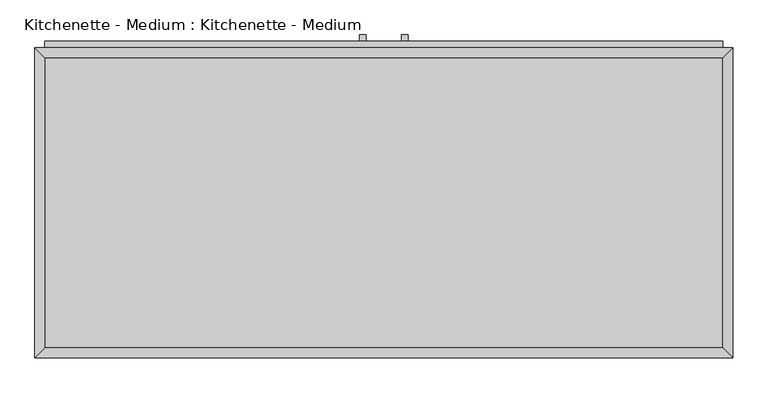
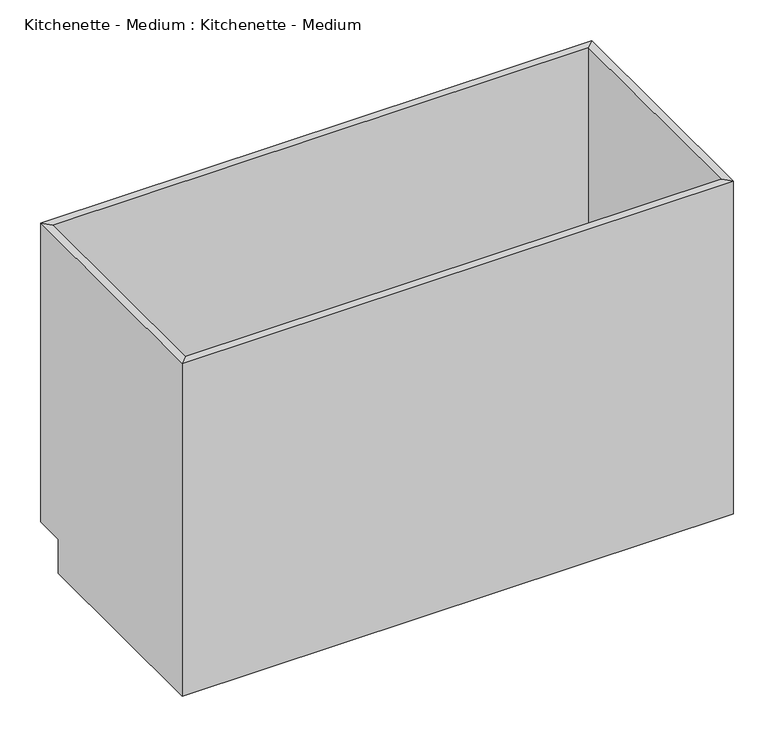
"""IFC4 building model written with IfcOpenShell, lengths in millimetres: proxy geometry, Kitchenette - Medium : Kitchenette - Medium."""

from ifc_helpers import new_model, si_unit, frame, origin, place, context, project, spatial, polyline, outline, extrude, faceted_brep, source, transform, mapped, element, save


def kitchenette_medium_kitchenette_medium_02f60b11(model_context):
    return source(origin(), model_context, "Body", "SolidModel", [
        faceted_brep([(685.4877049, 590.55, 876.3), (-648.0122951, 590.55, 876.3), (-648.0122951, 590.55, 88.9), (685.4877049, 590.55, 88.9), (704.5377049, 609.6, 876.3), (-667.0622951, 609.6, 876.3), (704.5377049, 609.6, 88.9), (-667.0622951, 609.6, 88.9), (-648.0122951, 19.05, 876.3), (-648.0122951, 19.05, 88.9), (-648.0122951, 533.4, 88.9), (-667.0622951, 0.0, 876.3), (-667.0622951, 533.4, 88.9), (-667.0622951, 533.4, 0.0), (-667.0622951, 0.0, 0.0), (685.4877049, 19.05, 876.3), (685.4877049, 19.05, 88.9), (704.5377049, 0.0, 876.3), (704.5377049, 0.0, 0.0), (685.4877049, 533.4, 88.9), (704.5377049, 533.4, 0.0), (704.5377049, 533.4, 88.9)], [[[0, 1, 2, 3]], [[0, 4, 5, 1]], [[4, 6, 7, 5]], [[2, 7, 6, 3]], [[1, 8, 9, 10, 2]], [[5, 11, 8, 1]], [[7, 12, 13, 14, 11, 5]], [[2, 10, 12, 7]], [[8, 15, 16, 9]], [[11, 17, 15, 8]], [[14, 18, 17, 11]], [[3, 19, 16, 15, 0]], [[0, 15, 17, 4]], [[4, 17, 18, 20, 21, 6]], [[6, 21, 19, 3]], [[10, 9, 16, 19]], [[18, 14, 13, 20]], [[13, 12, 10, 19, 21, 20]]]),
        extrude(outline(polyline([(-16.1872951, 635.0), (-16.1872951, 622.3), (-28.8872951, 622.3), (-28.8872951, 635.0), (-16.1872951, 635.0)])), frame((0.0, 0.0, 573.769895), z_axis=(0.0, 0.0, 1.0), x_axis=(1.0, 0.0, 0.0)), (0.0, 0.0, 1.0), 124.730105),
        extrude(outline(polyline([(66.3627049, 635.0), (66.3627049, 622.3), (53.6627049, 622.3), (53.6627049, 635.0), (66.3627049, 635.0)])), frame((0.0, 0.0, 573.769895), z_axis=(0.0, 0.0, 1.0), x_axis=(1.0, 0.0, 0.0)), (0.0, 0.0, 1.0), 124.730105),
        extrude(outline(polyline([(685.4877049, 19.05), (-648.0122951, 19.05), (-648.0122951, 590.55), (685.4877049, 590.55), (685.4877049, 19.05)])), frame((0.0, 0.0, 88.9), z_axis=(0.0, 0.0, 1.0), x_axis=(1.0, 0.0, 0.0)), (0.0, 0.0, 1.0), 19.05),
        extrude(outline(polyline([(9.2127049, 622.3), (9.2127049, 609.6), (-648.0122951, 609.6), (-648.0122951, 622.3), (9.2127049, 622.3)])), frame((0.0, 0.0, 107.95), z_axis=(0.0, 0.0, 1.0), x_axis=(1.0, 0.0, 0.0)), (0.0, 0.0, 1.0), 628.65),
        extrude(outline(polyline([(685.4877049, 622.3), (685.4877049, 609.6), (28.2627049, 609.6), (28.2627049, 622.3), (685.4877049, 622.3)])), frame((0.0, 0.0, 107.95), z_axis=(0.0, 0.0, 1.0), x_axis=(1.0, 0.0, 0.0)), (0.0, 0.0, 1.0), 628.65),
        extrude(outline(polyline([(685.4877049, 622.3), (685.4877049, 609.6), (-648.0122951, 609.6), (-648.0122951, 622.3), (685.4877049, 622.3)])), frame((0.0, 0.0, 755.65), z_axis=(0.0, 0.0, 1.0), x_axis=(1.0, 0.0, 0.0)), (0.0, 0.0, 1.0), 101.6),
    ])


if __name__ == "__main__":
    model = new_model("IFC4")
    model_context = context("Model", 3, world=origin())
    ifc_project = project(units=[si_unit("LENGTHUNIT", "METRE", prefix="MILLI")], contexts=[model_context])
    site = spatial("IfcSite", under=ifc_project)
    building = spatial("IfcBuilding", under=site)
    placement = place(None, origin())
    kitchenette_medium_kitchenette_medium_shape = kitchenette_medium_kitchenette_medium_02f60b11(model_context)
    element("IfcBuildingElementProxy", 1, Name="Kitchenette - Medium : Kitchenette - Medium", ObjectType="Kitchenette - Medium : Kitchenette - Medium", at=placement, inside=building, context=model_context, shape_type="MappedRepresentation", body=[
        mapped(kitchenette_medium_kitchenette_medium_shape, transform((0.0, 0.0, 0.0), x_axis=(1.0, 0.0, 0.0), y_axis=(0.0, 1.0, 0.0), z_axis=(0.0, 0.0, 1.0))),
    ])
    save(model, "model.ifc")

# Revit data of these elements
# Type "Kitchenette - Medium : Kitchenette - Medium"
#   Assembly Code = "E1090400"
#   Counter Length = 6' - 6"
#   Cabinet Width = 4' - 6"
#   Cabinet Height = 2' - 10 1/2"
#   Cabinet Depth = 2' - 0"
#   Toe Depth = 0' - 3"
#   Toe Height = 0' - 3 1/2"
#   Cabinet Material = Cabinets
#   Door/Drawer Material = Cabinets
#   Handle Material = Cabinets - Handles
#   Default Elevation = 0
# Element 1 (IfcBuildingElementProxy, "Kitchenette - Medium : Kitchenette - Medium")
#   Materials on its faces: "Cabinets", "Cabinets - Handles"
# Materials
#   "Cabinets": colour RGB 249 249 249, transparency 0
#   "Cabinets - Handles": class "Metal", colour RGB 57 57 57, transparency 0
